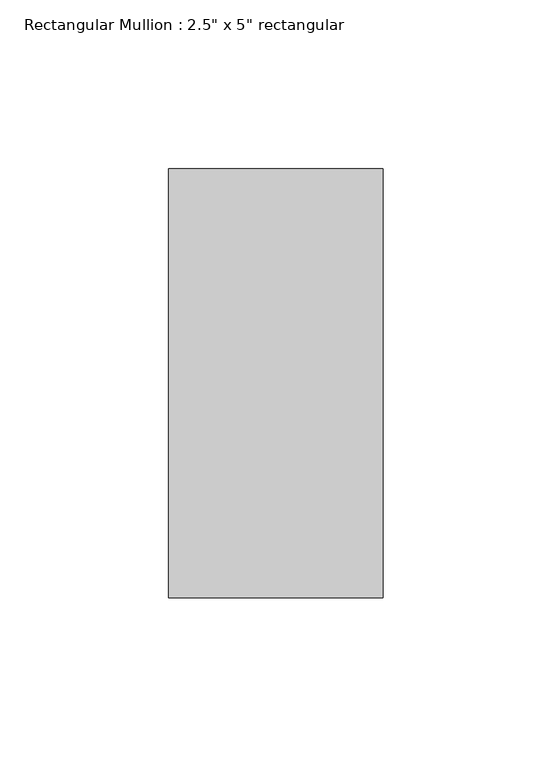
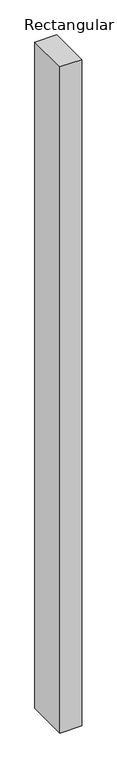
"""IFC4 building model written with IfcOpenShell, lengths in millimetres: member geometry."""

from ifc_helpers import new_model, si_unit, frame, origin, place, context, project, spatial, polyline, outline, extrude, source, transform, mapped, element, save


def member_8eaddbd8(model_context):
    return source(origin(), model_context, "Body", "SweptSolid", [
        extrude(outline(polyline([(0.0, 63.5), (0.0, -63.5), (-63.5, -63.5), (-63.5, 63.5), (0.0, 63.5)])), frame((0.0, 0.0, -2063.6147749), z_axis=(0.0, 0.0, 1.0), x_axis=(1.0, 0.0, 0.0)), (0.0, 0.0, 1.0), 2063.6147749),
    ])


if __name__ == "__main__":
    model = new_model("IFC4")
    model_context = context("Model", 3, world=origin())
    ifc_project = project(units=[si_unit("LENGTHUNIT", "METRE", prefix="MILLI")], contexts=[model_context])
    site = spatial("IfcSite", under=ifc_project)
    building = spatial("IfcBuilding", under=site)
    placement = place(None, origin())
    member_shape = member_8eaddbd8(model_context)
    element("IfcMember", 1, ObjectType="Rectangular Mullion : 2.5\" x 5\" rectangular", at=placement, inside=building, context=model_context, shape_type="MappedRepresentation", body=[
        mapped(member_shape, transform((0.0, 0.0, 0.0), x_axis=(1.0, 0.0, 0.0), y_axis=(0.0, 1.0, 0.0), z_axis=(0.0, 0.0, 1.0))),
    ])
    save(model, "model.ifc")

# Revit data of these elements
# Type "Rectangular Mullion : 2.5\" x 5\" rectangular"
#   built-in parameter 1007304 = 0.416667 (stored number, unit not read)
#   built-in parameter 1007301 = 0.104167 (stored number, unit not read)
#   built-in parameter 1007300 = 0.104167 (stored number, unit not read)
# Element 1 (IfcMember, "Rectangular Mullion : 2.5\" x 5\" rectangular")
#   Materials on its faces: "Aluminum"
# Materials
#   "Aluminum": class "Metal", colour RGB 247 247 247, transparency 0, Description = "Aluminum 6061", Cost = 0
